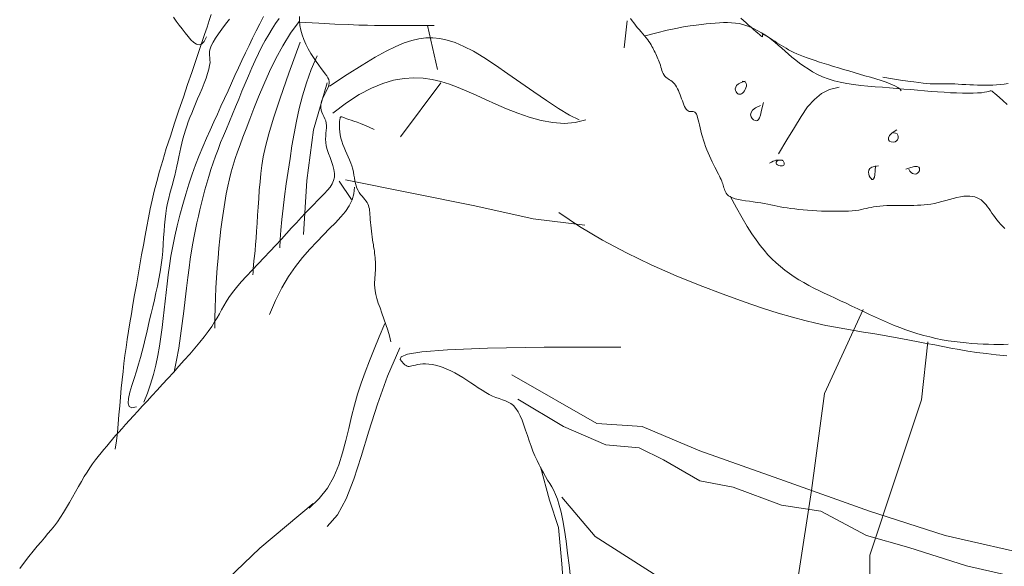
# Model space of a CAD drawing. Units: inches. Extents: x -17 to 1735, y -531 to 60.
# Tile 21 of 27: x 1734.799014 to 1734.803049, y -150.210609 to -150.208371. Entities that reach past the tile are written whole.
import ezdxf

# ---------------------------------------------------------------- set-up
doc = ezdxf.new("R2010")
doc.units = ezdxf.units.IN
doc.header["$MEASUREMENT"] = 0
doc.layers.add('A-FURN', color=242, linetype='Continuous', lineweight=18, true_color=0xcd2027)

# ---------------------------------------------------------------- blocks, each defined once
blk = doc.blocks.new('childrens_room_2')
for points in [[(73.33089, 54.3612), (73.3312, 54.36078), (73.3315, 54.36037), (73.33181, 54.35997), (73.33212, 54.35957), (73.33242, 54.35919), (73.33272, 54.35884), (73.33302, 54.35856), (73.3333, 54.35838), (73.33358, 54.35831), (73.33385, 54.3584), (73.33411, 54.35867), (73.33435, 54.35915)], [(73.33483, 54.36146), (73.33462, 54.36084), (73.3344, 54.36016), (73.33415, 54.3594), (73.33387, 54.35856), (73.33355, 54.35762), (73.3332, 54.35658), (73.33281, 54.35542), (73.33238, 54.35417), (73.33193, 54.35286), (73.33147, 54.35151), (73.33102, 54.35015), (73.33058, 54.34881), (73.33016, 54.34752), (73.32978, 54.34629), (73.32945, 54.34516), (73.32916, 54.3441), (73.32891, 54.34311), (73.32869, 54.34216), (73.32849, 54.34124), (73.3283, 54.34033), (73.32812, 54.33942), (73.32794, 54.33847), (73.32777, 54.33749), (73.32758, 54.33647), (73.3274, 54.33543), (73.32722, 54.33438), (73.32704, 54.33334), (73.32686, 54.33231), (73.32669, 54.3313), (73.32653, 54.33034), (73.32637, 54.32941), (73.32623, 54.32853), (73.3261, 54.32768), (73.32597, 54.32684), (73.32585, 54.32602), (73.32575, 54.32519), (73.32565, 54.32435), (73.32555, 54.32349), (73.32547, 54.3226), (73.32539, 54.32168), (73.32531, 54.32076), (73.32523, 54.31983), (73.32515, 54.31891), (73.32506, 54.318), (73.32496, 54.31712), (73.32484, 54.31627)], [(73.34028, 54.36124), (73.3399, 54.3605), (73.33952, 54.35976), (73.33914, 54.359), (73.33877, 54.35824), (73.3384, 54.35747), (73.33803, 54.35669), (73.33767, 54.35591), (73.3373, 54.35512), (73.33694, 54.35433), (73.33658, 54.35354), (73.33621, 54.35273), (73.33584, 54.35193), (73.33547, 54.35111), (73.33509, 54.35029), (73.33471, 54.34945), (73.33433, 54.34859), (73.33395, 54.34771), (73.33358, 54.34679), (73.33321, 54.34584), (73.33286, 54.34486), (73.33251, 54.34383), (73.33218, 54.34277), (73.33187, 54.34169), (73.33157, 54.34059), (73.3313, 54.3395), (73.33105, 54.33842), (73.33083, 54.33736), (73.33064, 54.33633), (73.33048, 54.33534), (73.33034, 54.33439), (73.33023, 54.33346), (73.33013, 54.33255), (73.33003, 54.33165), (73.32994, 54.33075), (73.32984, 54.32984), (73.32973, 54.32891), (73.3296, 54.32796), (73.32944, 54.32698), (73.32926, 54.326), (73.32905, 54.325), (73.32881, 54.32402), (73.32852, 54.32304), (73.3282, 54.32208), (73.32783, 54.32114)], [(73.34192, 54.36104), (73.34154, 54.36051), (73.34118, 54.35996), (73.34082, 54.35939), (73.34046, 54.35877), (73.34011, 54.35812), (73.33976, 54.35742), (73.33941, 54.35667), (73.33906, 54.3559), (73.33871, 54.3551), (73.33837, 54.35429), (73.33803, 54.35348), (73.33769, 54.35267), (73.33736, 54.35187), (73.33704, 54.35109), (73.33672, 54.35033), (73.33641, 54.34959), (73.3361, 54.34886), (73.33581, 54.34814), (73.33554, 54.34743), (73.33527, 54.34673), (73.33502, 54.34603), (73.33479, 54.34533), (73.33457, 54.34463), (73.33437, 54.34393), (73.33417, 54.34323), (73.33399, 54.34254), (73.33382, 54.34185), (73.33366, 54.34116), (73.3335, 54.34048), (73.33335, 54.3398), (73.3332, 54.33911), (73.33306, 54.33841), (73.33292, 54.33767), (73.33279, 54.33688), (73.33265, 54.33603), (73.33252, 54.33511), (73.33239, 54.33411), (73.33226, 54.33301), (73.33212, 54.33184), (73.33198, 54.3306), (73.33182, 54.32933), (73.33165, 54.32805), (73.33145, 54.32677), (73.33123, 54.32551), (73.33099, 54.3243)], [(73.34403, 54.36124), (73.34403, 54.36079), (73.34407, 54.36033), (73.34415, 54.35985), (73.34429, 54.35936), (73.34447, 54.35887), (73.34469, 54.35837), (73.34494, 54.35789), (73.34521, 54.35742), (73.34549, 54.35698), (73.34577, 54.35656), (73.34604, 54.35618), (73.34628, 54.35584), (73.34651, 54.35555), (73.3467, 54.3553), (73.34685, 54.35508), (73.34697, 54.35488), (73.34706, 54.35469), (73.34711, 54.35451), (73.34711, 54.35432), (73.34707, 54.35411), (73.34699, 54.35388), (73.34688, 54.35363), (73.34675, 54.35337), (73.34661, 54.3531), (73.34648, 54.35282), (73.34636, 54.35255), (73.34628, 54.35227), (73.34623, 54.35201), (73.34624, 54.35176), (73.34629, 54.35152), (73.34636, 54.3513), (73.34646, 54.35107), (73.34657, 54.35085), (73.34667, 54.35063), (73.34675, 54.35041), (73.34681, 54.35017), (73.34683, 54.34993), (73.34683, 54.34968), (73.3468, 54.34941), (73.34677, 54.34913), (73.34675, 54.34883), (73.34674, 54.34851), (73.34675, 54.34817), (73.34681, 54.34781), (73.34691, 54.34743), (73.34705, 54.34702), (73.3472, 54.34661), (73.34735, 54.34619), (73.34749, 54.34576), (73.34759, 54.34535), (73.34765, 54.34494), (73.34765, 54.34456), (73.34757, 54.3442), (73.34743, 54.34385), (73.34721, 54.34351), (73.34695, 54.34318), (73.34664, 54.34284), (73.34628, 54.34249), (73.3459, 54.34212), (73.3455, 54.34172), (73.34508, 54.34129), (73.34464, 54.34083), (73.34418, 54.34034), (73.3437, 54.33981), (73.3432, 54.33927), (73.34268, 54.33869), (73.34213, 54.33809), (73.34156, 54.33747), (73.34095, 54.33683), (73.34033, 54.33619), (73.33971, 54.33553), (73.3391, 54.33489), (73.33851, 54.33426), (73.33796, 54.33365), (73.33747, 54.33307), (73.33704, 54.33254), (73.33668, 54.33205), (73.33638, 54.3316), (73.33613, 54.33117), (73.3359, 54.33076), (73.33568, 54.33035), (73.33545, 54.32993), (73.33519, 54.32949), (73.33488, 54.32902), (73.33452, 54.32851), (73.33409, 54.32796), (73.33363, 54.32738), (73.33312, 54.32677), (73.33259, 54.32615), (73.33203, 54.32552), (73.33146, 54.32488), (73.33089, 54.32425), (73.33032, 54.32362), (73.32976, 54.32301), (73.32921, 54.32241), (73.32867, 54.32183), (73.32816, 54.32127), (73.32766, 54.32073), (73.32718, 54.32022), (73.32674, 54.31973), (73.32632, 54.31928), (73.32592, 54.31884), (73.32555, 54.31843), (73.32521, 54.31804), (73.32487, 54.31767), (73.32455, 54.3173), (73.32425, 54.31694), (73.32395, 54.31659), (73.32365, 54.31624), (73.32336, 54.31588), (73.32307, 54.31552), (73.32278, 54.31514), (73.32249, 54.31475), (73.3222, 54.31434), (73.32191, 54.31389), (73.32162, 54.31342), (73.32132, 54.31292), (73.32101, 54.31239), (73.32071, 54.31184), (73.3204, 54.31128), (73.32008, 54.31073), (73.31977, 54.31019), (73.31946, 54.30967), (73.31914, 54.30918), (73.31883, 54.30872), (73.31851, 54.3083), (73.31818, 54.30789), (73.31784, 54.30748), (73.31749, 54.30706), (73.31712, 54.30663), (73.31672, 54.30617), (73.3163, 54.30566), (73.31586, 54.3051), (73.31539, 54.3045), (73.3149, 54.30385)], [(73.37222, 54.30291), (73.37208, 54.30419), (73.37193, 54.30546), (73.37177, 54.30669), (73.3716, 54.30784), (73.37143, 54.30886), (73.37125, 54.30973), (73.37106, 54.31045), (73.37087, 54.31105), (73.37068, 54.31155), (73.37048, 54.31198), (73.37028, 54.31236), (73.37007, 54.31271), (73.36985, 54.31306), (73.36963, 54.31343), (73.36941, 54.31381), (73.36919, 54.31422), (73.36897, 54.31464), (73.36875, 54.31509), (73.36853, 54.31556), (73.36832, 54.31606), (73.36812, 54.31658), (73.36793, 54.31712), (73.36774, 54.31767), (73.36755, 54.31823), (73.36737, 54.31876), (73.36718, 54.31927), (73.36698, 54.31974), (73.36677, 54.32016), (73.36654, 54.32051), (73.3663, 54.32079), (73.36603, 54.32101), (73.36575, 54.32117), (73.36545, 54.3213), (73.36514, 54.32141), (73.36481, 54.32152), (73.36447, 54.32163), (73.36412, 54.32177), (73.36376, 54.32195), (73.3634, 54.32216), (73.36302, 54.32239), (73.36263, 54.32265), (73.36224, 54.32291), (73.36184, 54.32318), (73.36143, 54.32345), (73.36102, 54.32372), (73.36061, 54.32396), (73.36019, 54.32419), (73.35977, 54.32441), (73.35936, 54.3246), (73.35896, 54.32476), (73.35856, 54.3249), (73.35818, 54.325), (73.35782, 54.32508), (73.35747, 54.32512), (73.35715, 54.32514), (73.35685, 54.32513), (73.35657, 54.3251), (73.35632, 54.32506), (73.35609, 54.32501), (73.35589, 54.32497), (73.35572, 54.32492), (73.35557, 54.32489), (73.35545, 54.32487), (73.35534, 54.32487), (73.35523, 54.3249), (73.35512, 54.32496), (73.35499, 54.32505), (73.35484, 54.32519), (73.35467, 54.32537), (73.3545, 54.3256), (73.35459, 54.32586), (73.35525, 54.32613), (73.35677, 54.32638), (73.35944, 54.3266), (73.36359, 54.32677), (73.36949, 54.32686), (73.37746, 54.32686)], [(73.33673, 54.36099), (73.33633, 54.36046), (73.33595, 54.35994), (73.3356, 54.35945), (73.33528, 54.35899), (73.33502, 54.35857), (73.33483, 54.3582), (73.33471, 54.3579), (73.33465, 54.35764), (73.33464, 54.35741), (73.33465, 54.3572), (73.33468, 54.35698), (73.3347, 54.35675), (73.33471, 54.35648), (73.33467, 54.35616), (73.33459, 54.35577), (73.33446, 54.35533), (73.33429, 54.35484), (73.33409, 54.35432), (73.33388, 54.35378), (73.33365, 54.35323), (73.33342, 54.35269), (73.3332, 54.35217), (73.33299, 54.35167), (73.3328, 54.3512), (73.33261, 54.35074), (73.33244, 54.3503), (73.33229, 54.34986), (73.33214, 54.34943), (73.33201, 54.34899), (73.33189, 54.34855), (73.33177, 54.34809), (73.33167, 54.34762), (73.33156, 54.34714), (73.33147, 54.34665), (73.33137, 54.34616), (73.33127, 54.34568), (73.33116, 54.34519), (73.33105, 54.34472), (73.33092, 54.34425), (73.33079, 54.34378), (73.33066, 54.34332), (73.33053, 54.34285), (73.33041, 54.34236), (73.33029, 54.34186), (73.33019, 54.34133), (73.3301, 54.34078), (73.33003, 54.34019), (73.32997, 54.33957), (73.32993, 54.33893), (73.32988, 54.33826), (73.32984, 54.33757), (73.32978, 54.33687), (73.32971, 54.33615), (73.32963, 54.33543), (73.32952, 54.3347), (73.32939, 54.33396), (73.32924, 54.33323), (73.32908, 54.33251), (73.32892, 54.33179), (73.32875, 54.33108), (73.32858, 54.33038), (73.32842, 54.32971), (73.32826, 54.32904), (73.32812, 54.3284), (73.32797, 54.32775), (73.32781, 54.32711), (73.32765, 54.32646), (73.32747, 54.32579), (73.32727, 54.3251), (73.32705, 54.32438), (73.32681, 54.32363), (73.32656, 54.32288), (73.32636, 54.32218), (73.32622, 54.32155), (73.32619, 54.32105), (73.3263, 54.32071), (73.32657, 54.32058), (73.32705, 54.32068)], [(73.40472, 54.35496), (73.40573, 54.35479), (73.40659, 54.35465), (73.40733, 54.35454), (73.40795, 54.35445), (73.40847, 54.35438), (73.40892, 54.35433), (73.40932, 54.35429), (73.40967, 54.35426), (73.41001, 54.35425), (73.41033, 54.35424), (73.41064, 54.35424), (73.41094, 54.35424), (73.41125, 54.35424), (73.41156, 54.35424), (73.41189, 54.35424), (73.41223, 54.35424), (73.41259, 54.35422), (73.41297, 54.3542), (73.41337, 54.35418), (73.41378, 54.35416), (73.41419, 54.35414), (73.4146, 54.35412), (73.415, 54.35411), (73.4154, 54.3541), (73.41579, 54.35411), (73.41617, 54.35412), (73.41656, 54.35415), (73.41695, 54.35418), (73.41736, 54.35423), (73.41779, 54.35429)], [(73.38995, 54.36108), (73.39022, 54.36084), (73.3905, 54.3606), (73.39077, 54.36036), (73.39103, 54.36013), (73.39128, 54.3599), (73.39151, 54.3597), (73.39171, 54.35952), (73.39189, 54.35937), (73.39203, 54.35925), (73.39214, 54.35918), (73.3922, 54.35915), (73.39222, 54.35916), (73.39222, 54.35919), (73.39221, 54.35924), (73.3922, 54.3593), (73.3922, 54.35935), (73.39222, 54.35939), (73.39227, 54.35939), (73.39236, 54.35936), (73.39249, 54.3593), (73.39265, 54.35922), (73.39284, 54.3591), (73.39304, 54.35898), (73.39326, 54.35883), (73.39349, 54.35868), (73.39372, 54.35853), (73.39396, 54.35838), (73.39419, 54.35824), (73.39442, 54.35809), (73.39467, 54.35795), (73.39492, 54.3578), (73.3952, 54.35766), (73.39548, 54.35752), (73.39579, 54.35738), (73.39613, 54.35724), (73.39649, 54.3571), (73.39687, 54.35695), (73.39728, 54.35681), (73.3977, 54.35667), (73.39815, 54.35652), (73.39862, 54.35637), (73.3991, 54.35622), (73.39961, 54.35607), (73.40012, 54.35592), (73.40066, 54.35576), (73.4012, 54.3556), (73.40175, 54.35544), (73.40231, 54.35527), (73.40288, 54.3551), (73.40345, 54.35493), (73.40401, 54.35476), (73.40457, 54.35459), (73.40509, 54.35441), (73.40556, 54.35423), (73.40597, 54.35405), (73.4063, 54.35387), (73.40654, 54.35369), (73.40666, 54.35351)], [(73.41742, 54.33921), (73.41721, 54.33943), (73.417, 54.33965), (73.4168, 54.33988), (73.41661, 54.34012), (73.41642, 54.34035), (73.41625, 54.34059), (73.41609, 54.34082), (73.41594, 54.34105), (73.41579, 54.34127), (73.41564, 54.34148), (73.41549, 54.34168), (73.41533, 54.34186), (73.41516, 54.34203), (73.41498, 54.34218), (73.41478, 54.34231), (73.41456, 54.34241), (73.41432, 54.34249), (73.41406, 54.34255), (73.41379, 54.34258), (73.41349, 54.34258), (73.41316, 54.34256), (73.41282, 54.3425), (73.41245, 54.34243), (73.41207, 54.34233), (73.41168, 54.34223), (73.41128, 54.34212), (73.41089, 54.34201), (73.4105, 54.34191), (73.41012, 54.34182), (73.40975, 54.34175), (73.40939, 54.3417), (73.40904, 54.34166), (73.40869, 54.34164), (73.40834, 54.34162), (73.40798, 54.34161), (73.40761, 54.34161), (73.40723, 54.34161), (73.40682, 54.34161), (73.40641, 54.34161), (73.40599, 54.34161), (73.40557, 54.3416), (73.40516, 54.34159), (73.40477, 54.34157), (73.40441, 54.34154), (73.40407, 54.34151), (73.40378, 54.34146), (73.40351, 54.34141), (73.40326, 54.34136), (73.40302, 54.3413), (73.40277, 54.34124), (73.40251, 54.34118), (73.40223, 54.34113), (73.40192, 54.34109), (73.40156, 54.34105), (73.40117, 54.34103), (73.40074, 54.34101), (73.40029, 54.341), (73.39982, 54.341), (73.39933, 54.34101), (73.39884, 54.34102), (73.39835, 54.34103), (73.39786, 54.34106), (73.39737, 54.34108), (73.3969, 54.34112), (73.39644, 54.34115), (73.396, 54.34119), (73.39557, 54.34124), (73.39516, 54.34129), (73.39477, 54.34135), (73.39441, 54.34141), (73.39406, 54.34148), (73.39373, 54.34154), (73.39341, 54.34161), (73.39308, 54.34168), (73.39275, 54.34175), (73.3924, 54.34181), (73.39204, 54.34187), (73.39165, 54.34193), (73.39125, 54.34199), (73.39085, 54.34204), (73.39045, 54.3421), (73.39006, 54.34216), (73.3897, 54.34223), (73.38938, 54.34231), (73.3891, 54.3424), (73.38887, 54.3425), (73.38868, 54.34262), (73.38854, 54.34275), (73.38843, 54.34288), (73.38835, 54.34302), (73.38829, 54.34317), (73.38824, 54.34331), (73.3882, 54.34345), (73.38816, 54.34358), (73.38812, 54.34372), (73.38808, 54.34385), (73.38803, 54.34399), (73.38797, 54.34414), (73.3879, 54.3443), (73.38782, 54.34447), (73.38773, 54.34466), (73.38763, 54.34486), (73.38751, 54.34509), (73.38738, 54.34533), (73.38724, 54.34559), (73.3871, 54.34586), (73.38696, 54.34615), (73.38682, 54.34644), (73.38668, 54.34675), (73.38654, 54.34707), (73.38641, 54.3474), (73.38629, 54.34773), (73.38617, 54.34807), (73.38606, 54.3484), (73.38596, 54.34873), (73.38587, 54.34906), (73.38579, 54.34938), (73.38571, 54.34969), (73.38565, 54.34998), (73.38558, 54.35026), (73.38552, 54.35051), (73.38546, 54.35074), (73.3854, 54.35094), (73.38534, 54.3511), (73.38526, 54.35122), (73.38518, 54.35129), (73.38509, 54.35134), (73.38499, 54.35136), (73.38489, 54.35136), (73.38478, 54.35136), (73.38468, 54.35136), (73.38457, 54.35138), (73.38447, 54.35143), (73.38438, 54.3515), (73.38428, 54.35161), (73.3842, 54.35174), (73.38411, 54.3519), (73.38403, 54.35207), (73.38395, 54.35227), (73.38387, 54.35247), (73.38379, 54.35269), (73.38371, 54.3529), (73.38363, 54.35312), (73.38355, 54.35334), (73.38346, 54.35355), (73.38337, 54.35375), (73.38327, 54.35394), (73.38317, 54.35411), (73.38305, 54.35426), (73.38293, 54.35439), (73.3828, 54.35449), (73.38267, 54.35459), (73.38253, 54.35467), (73.3824, 54.35476), (73.38228, 54.35484), (73.38216, 54.35494), (73.38206, 54.35505), (73.38196, 54.35517), (73.38188, 54.35532), (73.38182, 54.35548), (73.38175, 54.35564), (73.3817, 54.35582), (73.38164, 54.356), (73.38159, 54.35618), (73.38153, 54.35636), (73.38147, 54.35653), (73.3814, 54.3567), (73.38133, 54.35687), (73.38126, 54.35703), (73.38119, 54.3572), (73.38111, 54.35736), (73.38103, 54.35751), (73.38095, 54.35767), (73.38087, 54.35783), (73.38079, 54.35799), (73.3807, 54.35815), (73.38061, 54.35831), (73.38051, 54.35848), (73.38039, 54.35866), (73.38026, 54.35884), (73.38011, 54.35904), (73.37994, 54.35924), (73.37976, 54.35945), (73.37957, 54.35967), (73.37938, 54.35989), (73.37918, 54.36012), (73.37899, 54.36035), (73.37881, 54.36058), (73.37864, 54.36082), (73.37849, 54.36106)], [(73.34397, 54.36075), (73.34309, 54.35952), (73.34229, 54.35822), (73.34156, 54.35688), (73.3409, 54.35553), (73.3403, 54.3542), (73.33976, 54.35291), (73.33928, 54.3517), (73.33885, 54.35058), (73.33847, 54.34959), (73.33813, 54.34871), (73.33783, 54.34792), (73.33756, 54.34718), (73.33731, 54.34648), (73.3371, 54.3458), (73.3369, 54.34511), (73.33672, 54.34439), (73.33655, 54.34362), (73.33639, 54.3428), (73.33624, 54.34193), (73.3361, 54.34103), (73.33597, 54.3401), (73.33585, 54.33913), (73.33574, 54.33815), (73.33564, 54.33715), (73.33554, 54.33613), (73.33546, 54.33511), (73.33538, 54.33408), (73.33532, 54.33304), (73.33527, 54.332), (73.33523, 54.33095), (73.33521, 54.3299), (73.3352, 54.32885)], [(73.344, 54.36067), (73.34604, 54.36056), (73.34771, 54.36047), (73.34908, 54.36041), (73.35019, 54.36036), (73.35109, 54.36034), (73.35183, 54.36033), (73.35246, 54.36032), (73.35303, 54.36032), (73.35359, 54.36032), (73.35415, 54.36032), (73.35471, 54.36032), (73.3553, 54.36032), (73.35592, 54.36032), (73.35657, 54.36032), (73.35727, 54.36032), (73.35803, 54.36032)], [(73.37811, 54.36082), (73.3778, 54.35799)], [(73.38001, 54.35925), (73.38122, 54.35956), (73.38228, 54.35982), (73.3832, 54.36002), (73.38399, 54.36017), (73.38469, 54.36028), (73.3853, 54.36036), (73.38586, 54.36043), (73.38636, 54.36048), (73.38685, 54.36053), (73.3873, 54.36057), (73.38775, 54.3606), (73.38817, 54.36062), (73.38858, 54.36062), (73.38899, 54.36061), (73.38939, 54.36057), (73.38978, 54.36051), (73.39017, 54.36041), (73.39057, 54.36029), (73.39096, 54.36014), (73.39134, 54.35997), (73.39173, 54.35978), (73.3921, 54.35957), (73.39247, 54.35934), (73.39283, 54.35909), (73.39318, 54.35883), (73.39352, 54.35855), (73.39386, 54.35826), (73.39421, 54.35797), (73.39456, 54.35766), (73.39491, 54.35735), (73.39528, 54.35704), (73.39567, 54.35673), (73.39607, 54.35641), (73.3965, 54.3561), (73.39695, 54.3558), (73.39743, 54.35551), (73.39793, 54.35524), (73.39847, 54.35499), (73.39905, 54.35477), (73.39966, 54.35457), (73.40031, 54.35441), (73.40099, 54.35428), (73.4017, 54.35418), (73.40243, 54.35409), (73.40318, 54.35402), (73.40393, 54.35395), (73.40469, 54.3539), (73.40544, 54.35384), (73.40618, 54.35378), (73.40692, 54.35371), (73.40764, 54.35365), (73.40836, 54.35358), (73.40906, 54.35352), (73.40976, 54.35346), (73.41044, 54.35341), (73.41112, 54.35337), (73.41178, 54.35333), (73.41242, 54.35331), (73.41304, 54.35329), (73.41361, 54.35329), (73.41414, 54.35329), (73.4146, 54.35331), (73.415, 54.35333), (73.41532, 54.35337), (73.41555, 54.35341), (73.41572, 54.35346), (73.41583, 54.3535), (73.4159, 54.35353), (73.41596, 54.35354), (73.41602, 54.35353), (73.4161, 54.35348), (73.41621, 54.35339), (73.41638, 54.35326), (73.4166, 54.35307), (73.41689, 54.35283), (73.41724, 54.35251), (73.41767, 54.35212)], [(73.35733, 54.36032), (73.35838, 54.35576)], [(73.34409, 54.35857), (73.34292, 54.35536), (73.342, 54.35276), (73.34131, 54.35069), (73.34082, 54.34905), (73.34047, 54.34774), (73.34024, 54.34668), (73.3401, 54.34577), (73.34, 54.34493), (73.33991, 54.34407), (73.33984, 54.3432), (73.33978, 54.34232), (73.33972, 54.34144), (73.33966, 54.34058), (73.33961, 54.33975), (73.33955, 54.33895), (73.3395, 54.33821), (73.33944, 54.33753), (73.33939, 54.33691), (73.33933, 54.33635), (73.33928, 54.33585), (73.33924, 54.3354), (73.33921, 54.33501), (73.33919, 54.33467), (73.33918, 54.33439)], [(73.34715, 54.35401), (73.34899, 54.35521), (73.35056, 54.35621), (73.3519, 54.35701), (73.35305, 54.35765), (73.35405, 54.35814), (73.35493, 54.3585), (73.35572, 54.35875), (73.35645, 54.35892), (73.35717, 54.35902), (73.35789, 54.35904), (73.35863, 54.35897), (73.3594, 54.35881), (73.36023, 54.35854), (73.36113, 54.35815), (73.36212, 54.35764), (73.36321, 54.35699), (73.36442, 54.3562), (73.36571, 54.35531), (73.36705, 54.35437), (73.3684, 54.35342), (73.36972, 54.35251), (73.37097, 54.35169), (73.37212, 54.35101), (73.37312, 54.35051)], [(73.34585, 54.35717), (73.34524, 54.35575), (73.34474, 54.35437), (73.34433, 54.35302), (73.34398, 54.35169), (73.3437, 54.35038), (73.34345, 54.34909), (73.34324, 54.34779), (73.34304, 54.34648), (73.34284, 54.34516), (73.34265, 54.34384), (73.34247, 54.34255), (73.34231, 54.34131), (73.34218, 54.34013), (73.34208, 54.33904), (73.34201, 54.33805), (73.34199, 54.33719)], [(73.3469, 54.35437), (73.34549, 54.34946), (73.34479, 54.3442), (73.34444, 54.33859)], [(73.3475, 54.35121), (73.34891, 54.35228), (73.35024, 54.35314), (73.3515, 54.3538), (73.35269, 54.35429), (73.35382, 54.35462), (73.3549, 54.35481), (73.35592, 54.35487), (73.35689, 54.35483), (73.35783, 54.3547), (73.35874, 54.35449), (73.35963, 54.35422), (73.36053, 54.35388), (73.36145, 54.3535), (73.3624, 54.35307), (73.36339, 54.35262), (73.36444, 54.35214), (73.36556, 54.35166), (73.36673, 54.3512), (73.36794, 54.35078), (73.36916, 54.35045), (73.37038, 54.35022), (73.37158, 54.35014), (73.37273, 54.35022), (73.37383, 54.35051)], [(73.35873, 54.35436), (73.35452, 54.34875)], [(73.39041, 54.35452), (73.39, 54.35439), (73.38971, 54.35424), (73.38952, 54.35407), (73.38942, 54.3539), (73.38938, 54.35373), (73.3894, 54.35357), (73.38946, 54.35343), (73.38954, 54.35332), (73.38964, 54.35323), (73.38973, 54.35319), (73.38983, 54.35317), (73.38994, 54.35318), (73.39004, 54.35323), (73.39014, 54.3533), (73.39024, 54.3534), (73.39033, 54.35353), (73.39042, 54.35367), (73.39048, 54.35384), (73.39053, 54.354), (73.39054, 54.35416), (73.39051, 54.3543), (73.39043, 54.35442), (73.3903, 54.35449), (73.3901, 54.35452)], [(73.40018, 54.35389), (73.3992, 54.35367), (73.39836, 54.35325), (73.39761, 54.35264), (73.39691, 54.35185), (73.39623, 54.35087), (73.39553, 54.34973), (73.39476, 54.34842), (73.39388, 54.34696)], [(73.38883, 54.34256), (73.3895, 54.34135), (73.39009, 54.34031), (73.39062, 54.33943), (73.3911, 54.33867), (73.39154, 54.33802), (73.39196, 54.33745), (73.39237, 54.33695), (73.39278, 54.33649), (73.3932, 54.33606), (73.39363, 54.33565), (73.39408, 54.33526), (73.39454, 54.33489), (73.39502, 54.33454), (73.3955, 54.3342), (73.396, 54.33388), (73.39651, 54.33358), (73.39702, 54.33329), (73.39755, 54.33302), (73.39809, 54.33275), (73.39863, 54.33249), (73.39919, 54.33223), (73.39976, 54.33197), (73.40033, 54.3317), (73.40092, 54.33143), (73.40152, 54.33115), (73.40212, 54.33086), (73.40273, 54.33057), (73.40335, 54.33028), (73.40397, 54.32999), (73.4046, 54.32971), (73.40523, 54.32944), (73.40586, 54.32917), (73.40649, 54.32892), (73.40712, 54.32869), (73.40775, 54.32847), (73.40838, 54.32827), (73.40901, 54.32809), (73.40964, 54.32793), (73.41027, 54.32778), (73.41091, 54.32765), (73.41154, 54.32754), (73.41216, 54.32745), (73.41279, 54.32738), (73.4134, 54.32732), (73.41401, 54.32727), (73.4146, 54.32723), (73.41518, 54.3272), (73.41574, 54.32718), (73.41628, 54.32716), (73.4168, 54.32715), (73.4173, 54.32715), (73.41778, 54.32717)], [(73.39199, 54.352), (73.39149, 54.35176), (73.39118, 54.35151), (73.39102, 54.35127), (73.39097, 54.35104), (73.39102, 54.35083), (73.39113, 54.35065), (73.39128, 54.35052), (73.39144, 54.35043), (73.39157, 54.3504), (73.39169, 54.35044), (73.3918, 54.35054), (73.3919, 54.35072), (73.39199, 54.35099), (73.39209, 54.35134), (73.39219, 54.35178), (73.3923, 54.35232)], [(73.35352, 54.32744), (73.35338, 54.32804), (73.35321, 54.32864), (73.35302, 54.32924), (73.35281, 54.32983), (73.3526, 54.3304), (73.3524, 54.33095), (73.35222, 54.33146), (73.35208, 54.33193), (73.35197, 54.33235), (73.3519, 54.33272), (73.35185, 54.33305), (73.35184, 54.33336), (73.35184, 54.33363), (73.35185, 54.33389), (73.35187, 54.33413), (73.35189, 54.33437), (73.35191, 54.3346), (73.35192, 54.33484), (73.35193, 54.33507), (73.35193, 54.33531), (73.35193, 54.33554), (73.35192, 54.33576), (73.35191, 54.33599), (73.35189, 54.33621), (73.35187, 54.33642), (73.35184, 54.33663), (73.35181, 54.33685), (73.35178, 54.33706), (73.35174, 54.33729), (73.35171, 54.33753), (73.35167, 54.33778), (73.35163, 54.33804), (73.35159, 54.33833), (73.35155, 54.33863), (73.35151, 54.33893), (73.35148, 54.33924), (73.35144, 54.33955), (73.35141, 54.33985), (73.35139, 54.34014), (73.35137, 54.3404), (73.35135, 54.34065), (73.35133, 54.34087), (73.35131, 54.34107), (73.35129, 54.34126), (73.35125, 54.34144), (73.3512, 54.34161), (73.35114, 54.34177), (73.35105, 54.34193), (73.35094, 54.34208), (73.35081, 54.34224), (73.35067, 54.34241), (73.35053, 54.34258), (73.35038, 54.34276), (73.35024, 54.34296), (73.35011, 54.34317), (73.35, 54.3434), (73.34991, 54.34364), (73.34984, 54.3439), (73.34979, 54.34418), (73.34974, 54.34447), (73.34969, 54.34477), (73.34963, 54.34508), (73.34956, 54.34539), (73.34947, 54.34571), (73.34936, 54.34602), (73.34924, 54.34634), (73.3491, 54.34665), (73.34895, 54.34697), (73.3488, 54.34729), (73.34866, 54.34762), (73.34853, 54.34794), (73.34842, 54.34828), (73.34834, 54.34861), (73.34827, 54.34895), (73.34823, 54.34927), (73.3482, 54.34958), (73.34819, 54.34987), (73.34819, 54.35013), (73.3482, 54.35035), (73.34821, 54.35053), (73.34824, 54.35067), (73.34827, 54.35076), (73.34831, 54.35081), (73.34836, 54.35083), (73.34844, 54.35082), (73.34853, 54.35079), (73.34865, 54.35075), (73.34879, 54.35069), (73.34896, 54.35063), (73.34917, 54.35056), (73.34941, 54.35048), (73.34969, 54.35038), (73.35001, 54.35026), (73.35038, 54.35012), (73.3508, 54.34995), (73.35126, 54.34975), (73.35178, 54.34951)], [(73.40618, 54.34948), (73.4057, 54.34915), (73.40542, 54.34887), (73.40531, 54.34863), (73.40533, 54.34844), (73.40544, 54.3483), (73.40562, 54.34822), (73.40582, 54.34819), (73.40602, 54.34822), (73.40617, 54.34831), (73.40628, 54.34844), (73.40634, 54.34859), (73.40635, 54.34876), (73.40631, 54.34891), (73.40622, 54.34904), (73.40607, 54.34913), (73.40586, 54.34917)], [(73.39388, 54.34633), (73.3937, 54.34622), (73.39362, 54.3461), (73.39362, 54.346), (73.39368, 54.3459), (73.39379, 54.34582), (73.39392, 54.34576), (73.39406, 54.34572), (73.39419, 54.34571), (73.3943, 54.34572), (73.39437, 54.34576), (73.39443, 54.34581), (73.39446, 54.34588), (73.39447, 54.34596), (73.39446, 54.34604), (73.39444, 54.34611), (73.3944, 54.34618), (73.39436, 54.34623), (73.39431, 54.34627), (73.39425, 54.3463), (73.39418, 54.34632), (73.39412, 54.34633), (73.39405, 54.34633), (73.39398, 54.34633), (73.39391, 54.34633), (73.39384, 54.34633), (73.39376, 54.34633), (73.39368, 54.34632), (73.39359, 54.3463), (73.39347, 54.34626), (73.39333, 54.3462), (73.39315, 54.34612), (73.39293, 54.34602)], [(73.40428, 54.34571), (73.40387, 54.34567), (73.40358, 54.34558), (73.40339, 54.34544), (73.40329, 54.34526), (73.40325, 54.34507), (73.40328, 54.34487), (73.40333, 54.34469), (73.40342, 54.34452), (73.40351, 54.3444), (73.4036, 54.34432), (73.4037, 54.34431), (73.40378, 54.34438), (73.40386, 54.34454), (73.40392, 54.3448), (73.40395, 54.34519), (73.40397, 54.34571)], [(73.40744, 54.34539), (73.40756, 54.34518), (73.4077, 54.34503), (73.40784, 54.34493), (73.40798, 54.34488), (73.40812, 54.34487), (73.40825, 54.3449), (73.40836, 54.34497), (73.40846, 54.34508), (73.40854, 54.34521), (73.40857, 54.34535), (73.40856, 54.34548), (73.40847, 54.34559), (73.4083, 54.34565), (73.40803, 54.34565), (73.40764, 54.34557), (73.40712, 54.34539)], [(73.34816, 54.34413), (73.34942, 54.34224)], [(73.3488, 54.34426), (73.36227, 54.34156), (73.36834, 54.34022), (73.37372, 54.33955)], [(73.34974, 54.3435), (73.34967, 54.34282), (73.34949, 54.34218), (73.34919, 54.34158), (73.3488, 54.34099), (73.34832, 54.34041), (73.34778, 54.33981), (73.34716, 54.3392), (73.34651, 54.33854), (73.34581, 54.33783), (73.34509, 54.33706), (73.34435, 54.33621), (73.34362, 54.33526), (73.34289, 54.33421), (73.34219, 54.33304), (73.34153, 54.33173), (73.34091, 54.33027)], [(73.37103, 54.34089), (73.37318, 54.33941), (73.37555, 54.338), (73.37806, 54.33668), (73.38064, 54.33544), (73.38322, 54.3343), (73.38574, 54.33327), (73.38812, 54.33237), (73.39029, 54.33158), (73.3922, 54.33093), (73.39386, 54.3304), (73.39532, 54.32998), (73.39661, 54.32964), (73.39776, 54.32936), (73.39882, 54.32914), (73.39982, 54.32895), (73.40079, 54.32878), (73.40176, 54.32861), (73.40274, 54.32844), (73.40371, 54.32828), (73.40469, 54.32811), (73.40565, 54.32794), (73.4066, 54.32777), (73.40752, 54.3276), (73.40842, 54.32743), (73.40929, 54.32727), (73.41014, 54.3271), (73.41098, 54.32694), (73.41183, 54.32678), (73.41269, 54.32662), (73.41358, 54.32647), (73.41451, 54.32633), (73.41549, 54.3262), (73.41654, 54.32608), (73.41763, 54.32597)], [(73.40269, 54.3308), (73.39865, 54.32205), (73.3973, 54.31196), (73.39596, 54.30321), (73.39596, 54.30119), (73.39596, 54.30119)], [(73.35289, 54.32933), (73.35232, 54.32796), (73.35179, 54.32668), (73.35131, 54.32546), (73.35086, 54.32428), (73.35045, 54.32313), (73.35007, 54.32199), (73.34973, 54.32083), (73.34942, 54.31965), (73.34914, 54.31841), (73.34884, 54.31715), (73.34851, 54.31588), (73.3481, 54.31462), (73.34758, 54.31339), (73.34692, 54.31222), (73.34607, 54.31112), (73.34501, 54.31012)], [(73.35447, 54.32681), (73.35318, 54.32386), (73.35213, 54.32094), (73.35124, 54.31814), (73.35045, 54.31551), (73.34968, 54.31314), (73.34888, 54.31109), (73.34797, 54.30943), (73.3469, 54.30823)], [(73.40943, 54.32743), (73.40876, 54.32138), (73.40606, 54.3133), (73.40337, 54.30523), (73.40337, 54.30052), (73.40337, 54.29917), (73.40337, 54.29716)], [(73.36613, 54.32398), (73.37496, 54.31894), (73.37969, 54.31862), (73.38568, 54.3161), (73.39451, 54.31296), (73.40334, 54.30981), (73.41122, 54.30729), (73.42099, 54.30508), (73.42667, 54.30414), (73.43045, 54.30414), (73.43298, 54.30571), (73.43676, 54.30603), (73.44023, 54.3076), (73.44117, 54.30823)], [(73.36676, 54.32146), (73.37149, 54.31862), (73.37591, 54.31673), (73.37938, 54.31642), (73.3819, 54.31516), (73.38568, 54.31296), (73.38915, 54.31233), (73.39419, 54.31044), (73.39829, 54.30981), (73.40302, 54.30729), (73.40744, 54.30603), (73.41343, 54.30414), (73.41753, 54.30319), (73.42604, 54.30225), (73.43014, 54.30256), (73.43235, 54.30319), (73.43361, 54.30414), (73.43455, 54.30445), (73.4355, 54.30445), (73.43581, 54.30445), (73.43644, 54.30477), (73.43834, 54.30477), (73.43999, 54.30587)], [(73.3691, 54.31443), (73.37005, 54.31097), (73.37099, 54.30813), (73.37131, 54.30435), (73.37162, 54.30057), (73.37194, 54.29743), (73.37194, 54.29428), (73.37005, 54.28987)], [(73.37131, 54.31128), (73.37478, 54.30719), (73.38171, 54.30278), (73.3896, 54.30089), (73.39559, 54.30089), (73.40252, 54.29774), (73.40694, 54.29743), (73.41261, 54.29743), (73.41892, 54.29743), (73.42302, 54.29837), (73.42712, 54.29963), (73.43027, 54.30089), (73.43216, 54.30341)], [(73.34543, 54.31061), (73.3399, 54.30598), (73.33493, 54.30121), (73.33052, 54.29635), (73.32665, 54.29144), (73.32332, 54.28652), (73.32051, 54.28166), (73.31823, 54.27689), (73.31646, 54.27226)]]:
    blk.add_lwpolyline(points)

msp = doc.modelspace()

# ---------------------------------------------------------------- block references
at = {"layer": 'A-FURN', "xscale": 0.0393700787401575, "yscale": 0.0393700787401575, "zscale": 0.0393700787401575}
msp.add_blockref('childrens_room_2', (1731.9126009, -152.348565), dxfattribs=at)

doc.saveas('drawing.dxf')
